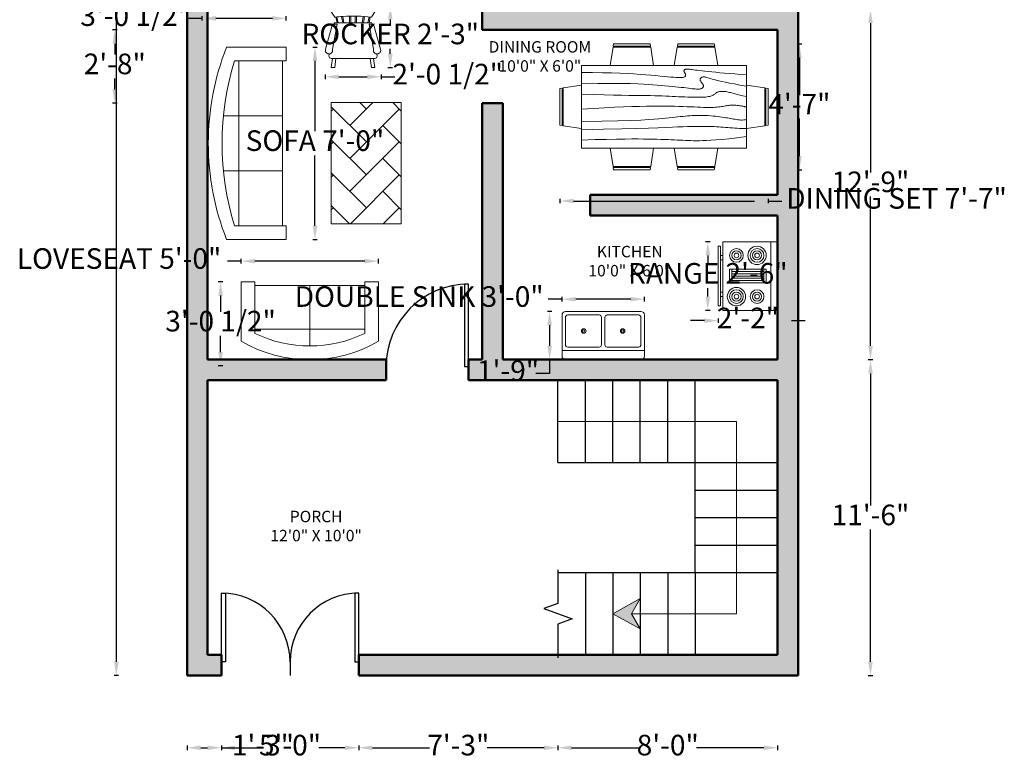
# Model space of a CAD drawing. Units: inches. Extents: x -31 to 401, y -19 to 637.
# Tile 1 of 2: x -29 to 401, y -19 to 305. Entities that reach past the tile are written whole.
import ezdxf

# ---------------------------------------------------------------- set-up
doc = ezdxf.new("R2010")
doc.units = ezdxf.units.IN
for name, color, linetype, lineweight in [('A-ANNO-DIMS', 2, 'Continuous', 18), ('A-ANNO-SYMB', 7, 'Continuous', 18), ('A-AREA-IDEN', 7, 'Continuous', 25), ('A-DOOR', 4, 'Continuous', 25), ('A-EQPM', 8, 'Continuous', 18), ('A-FLOR-FIXT', 9, 'Continuous', 18), ('A-FLOR-STRS', 7, 'Continuous', 25), ('A-FURN', 8, 'Continuous', 18), ('A-FURN-PATT', 9, 'Continuous', 13), ('A-WALL', 7, 'Continuous', 50), ('A-WALL-PATT', 252, 'Continuous', 13)]:
    doc.layers.add(name, color=color, linetype=linetype, lineweight=lineweight)
doc.styles.get("Standard").update_dxf_attribs({"font": 'arial.ttf'})
doc.dimstyles.new('ISO-25', dxfattribs={"dimtxt": 9, "dimasz": 6, "dimexe": 1, "dimexo": 2, "dimtad": 0, "dimtih": 1, "dimtoh": 1, "dimdec": 1, "dimlunit": 3, "dimtxsty": 'Standard', "dimcen": 2.5, "dimadec": 0, "dimazin": 0, "dimtfac": 1, "dimtdec": 1, "dimtmove": 0, "dimatfit": 3, "dimfxl": 1, "dimfxlon": 1, "dimarcsym": 0})

# ---------------------------------------------------------------- blocks, each defined once
blk = doc.blocks.new('*U8')
for p, q in [((0, 0), (0, -6)), ((30, 0), (30, -6))]:
    blk.add_line(p, q)
blk.add_lwpolyline([(0, 0), (0, 30), (1.75, 30), (1.75, 0)], close=True)
blk.add_arc((0, 0), 30, 0, 90)
blk = doc.blocks.new('*U7')
for p, q in [((-30, 0), (-30, -6)), ((0, 0), (0, -6))]:
    blk.add_line(p, q)
blk.add_lwpolyline([(0, 0), (0, 30), (-1.75, 30), (-1.75, 0)], close=True)
blk.add_arc((0, 0), 30, 90, 180)
blk = doc.blocks.new('*U9')
for p, q in [((0, 0), (0, -6)), ((-36, 0), (-36, -6))]:
    blk.add_line(p, q)
blk.add_lwpolyline([(0, 0), (0, 36), (-1.75, 36), (-1.75, 0)], close=True)
blk.add_arc((0, 0), 36, 90, 180)
blk = doc.blocks.new('Sofa - Roundback 7 ft.')
for p, q in [((-12.00002, -32.4421), (-12.00003, -6.5971)), ((11.99997, -32.4421), (11.99998, -6.5971)), ((-36.000027, -34), (-36.000027, -11.4696)), ((35.99998, -34), (35.99998, -11.4696)), ((-35.999844, -13.3819), (35.9998, -13.3819)), ((-36.000027, -32.4421), (35.99998, -32.4421))]:
    blk.add_line(p, q)
for points in [[(-36.000027, -34), (-42.000027, -34), (-42.000027, -8)], [(41.99998, -8), (41.99998, -34), (35.99998, -34)]]:
    blk.add_lwpolyline(points)
for centre, radius, start, end in [((0, -114.25), 114.25, 68.43141, 111.5686), ((-0.00001, -127.1968), 121.1968, 72.72033, 107.2797)]:
    blk.add_arc(centre, radius, start, end)
blk = doc.blocks.new('Chair - Rocking')
for p, q in [((-8, -4.5), (-10, -1.5)), ((-4.5, -7), (-4.96674, -4.19951)), ((-4, -7), (-4.40532, -4.16272)), ((-1.5, -4.05012), (-1.5, -7)), ((-1, -7), (-1, -4.05012)), ((1, -7), (1, -4.04655)), ((1.5, -4.05012), (1.5, -7)), ((4, -7), (4.40187, -4.18694)), ((4.5, -7), (4.96761, -4.19437)), ((8, -4.5), (10, -1.5)), ((-9, -7.5), (-12, -18.49999)), ((-7, -7.5), (-9, -7.5)), ((-9, -18.49999), (-7, -7.5)), ((-8.23428, -6.99939), (-8.3093, -7.47958)), ((-8.23041, -7), (8.23915, -7)), ((-7.5, -4.5), (-7, -7)), ((-6.5, -7), (-7.02225, -4.43)), ((6.5, -7), (7, -4.4057)), ((7.5, -4.5), (7, -7)), ((7, -7.5), (9, -7.5)), ((9, -18.49999), (7, -7.5)), ((8.31071, -7.48854), (8.23449, -7.00073)), ((9, -7.5), (12, -18.49999)), ((-10.36644, -20.64523), (-10.5, -21.49999)), ((10.5, -21.49999), (10.3575, -20.58798)), ((-9, -22.49999), (-9.5, -26.49999)), ((0, -22.49999), (-9.5, -22.49999)), ((-8, -26.49999), (-7.5, -22.49999)), ((0, -22.49999), (9.5, -22.49999)), ((8, -26.49999), (7.5, -22.49999)), ((9, -22.49999), (9.5, -26.49999)), ((-9.5, -26.49999), (-8, -26.49999)), ((9.5, -26.49999), (8, -26.49999))]:
    blk.add_line(p, q)
for centre, radius, start, end in [((0, -34.08333), 34.08333, 72.93847, 107.0615), ((0, -68.25004), 64.25, 93.92211, 97.15267), ((0, -68.25004), 64.25, 82.84733, 93.92211), ((-10.5, -18.99999), 1.58114, 161.5651, 18.43495), ((-9.5, -21.49999), 1, 180, 270), ((10.5, -18.99999), 1.58114, 161.5651, 18.43495), ((9.5, -21.49999), 1, 270, 0)]:
    blk.add_arc(centre, radius, start, end)
blk = doc.blocks.new('Sofa - Roundback Loveseat 5 ft.')
for p, q in [((0, -32.44198), (0, -5.99998)), ((-24, -33.99998), (-24, -11.46958)), ((24.00004, -33.99998), (24.00004, -11.46958)), ((-23.9998, -13.38178), (23.99986, -13.38178)), ((-24, -32.44198), (24.00004, -32.44198))]:
    blk.add_line(p, q)
for points in [[(-24, -33.99998), (-30, -33.99998), (-30, -7.99998)], [(30.00004, -7.99998), (30.00004, -33.99998), (24.00004, -33.99998)]]:
    blk.add_lwpolyline(points)
for centre, radius, start, end in [((0, -60.24998), 60.24998, 60.13715, 119.8628), ((0, -61.38438), 55.38444, 64.32083, 115.6792)]:
    blk.add_arc(centre, radius, start, end)
blk = doc.blocks.new('Dining Set - 36 x 72 in.')
for p, q in [((-22.2343, 26.00059), (-23.4847, 17.99762)), ((-22.2304, 26), (-5.7608, 26)), ((-22, 27.5), (-22.1562, 26.50042)), ((-5.8416, 26.5), (-22.1534, 26.5)), ((-22, 27.5), (-6, 27.5)), ((-5.8437, 26.49966), (-6, 27.5)), ((-4.5152, 17.99762), (-5.7655, 25.99926)), ((5.7657, 26.00059), (4.5153, 17.99762)), ((5.7696, 26), (22.2392, 26)), ((6, 27.5), (5.8438, 26.50042)), ((22.1584, 26.5), (5.8466, 26.5)), ((6, 27.5), (22, 27.5)), ((22.1563, 26.49966), (22, 27.5)), ((23.4848, 17.99762), (22.2345, 25.99926)), ((36, 18), (-36, 18)), ((-36, 18), (-36, -18)), ((36, -18), (36, 18)), ((-44.0006, 8.23428), (-35.9976, 9.48474)), ((44.0006, 8.23428), (35.9976, 9.48474)), ((-45.5, 8), (-44.5004, 8.15617)), ((-45.5, 8), (-45.5, -8)), ((-44.5, -8.15843), (-44.5, 8.15338)), ((-44, 8.23041), (-44, -8.23915)), ((44, 8.23041), (44, -8.23915)), ((44.5, -8.15843), (44.5, 8.15338)), ((45.5, 8), (44.5005, 8.15617)), ((45.5, 8), (45.5, -8)), ((-44.4997, -8.15631), (-45.5, -8)), ((-35.9976, -9.48476), (-43.9993, -8.2345)), ((35.9976, -9.48476), (43.9993, -8.2345)), ((44.4997, -8.15631), (45.5, -8)), ((-36, -18), (36, -18)), ((-22.2343, -26.0006), (-23.4847, -17.99762)), ((-4.5152, -17.99762), (-5.7655, -25.99928)), ((5.7657, -26.0006), (4.5153, -17.99762)), ((23.4848, -17.99762), (22.2345, -25.99928)), ((-22.2304, -26), (-5.7608, -26)), ((-22, -27.5), (-22.1562, -26.50044)), ((-5.8416, -26.5), (-22.1534, -26.5)), ((-22, -27.5), (-6, -27.5)), ((-5.8437, -26.49967), (-6, -27.5)), ((5.7696, -26), (22.2392, -26)), ((6, -27.5), (5.8438, -26.50044)), ((22.1584, -26.5), (5.8466, -26.5)), ((6, -27.5), (22, -27.5)), ((22.1563, -26.49967), (22, -27.5))]:
    blk.add_line(p, q)
for points in [[(-36, 15), (-31.1772, 14.97754), (-26.8079, 14.91406), (-22.8538, 14.81543), (-19.276, 14.6875), (-16.0362, 14.53613), (-13.0957, 14.36718), (-10.4159, 14.18652), (-7.9583, 14), (-5.6904, 13.81315), (-3.6035, 13.63021), (-1.6954, 13.45508), (0.0365, 13.29166), (1.5945, 13.14388), (2.9811, 13.01562), (4.1988, 12.9108), (5.25, 12.83333), (6.1393, 12.78613), (6.8802, 12.76823), (7.4883, 12.77767), (7.9792, 12.8125), (8.3685, 12.87077), (8.6719, 12.95052), (8.9049, 13.0498), (9.0833, 13.16666), (9.2205, 13.29899), (9.3216, 13.44401), (9.3895, 13.59879), (9.4271, 13.76041), (9.4373, 13.92594), (9.4232, 14.09245), (9.3875, 14.257), (9.3333, 14.41666), (9.2638, 14.56917), (9.1836, 14.71484), (9.0975, 14.85465), (9.0104, 14.98958), (8.9272, 15.1206), (8.8529, 15.2487), (8.7922, 15.37483), (8.75, 15.5), (8.7305, 15.62467), (8.7344, 15.74739), (8.7617, 15.86621), (8.8125, 15.97916), (8.8867, 16.08431), (8.9844, 16.17968), (9.1055, 16.26334), (9.25, 16.33333), (9.4189, 16.38802), (9.6172, 16.42708), (9.8506, 16.45052), (10.125, 16.45833), (10.4463, 16.45052), (10.8203, 16.42708), (11.2529, 16.38802), (11.75, 16.33333), (12.3184, 16.26318), (12.9694, 16.17838), (13.7151, 16.07991), (14.5677, 15.96875), (15.5395, 15.84586), (16.6426, 15.71224), (17.8893, 15.56884), (19.2917, 15.41666), (20.859, 15.25667), (22.5879, 15.08984), (24.4721, 14.91715), (26.5052, 14.73958), (28.6809, 14.5581), (30.9929, 14.3737), (33.4347, 14.18733), (36, 14)], [(-36, 10), (-28.9766, 10.14274), (-23.1725, 10.20442), (-18.4241, 10.19775), (-14.5677, 10.13541), (-11.4399, 10.03011), (-8.877, 9.89453), (-6.7154, 9.74137), (-4.7917, 9.58333), (-2.9698, 9.43082), (-1.2246, 9.28515), (0.4415, 9.14534), (2.026, 9.01041), (3.5266, 8.87939), (4.9408, 8.7513), (6.266, 8.62516), (7.5, 8.5), (8.6411, 8.37549), (9.6914, 8.2539), (10.6538, 8.13818), (11.5312, 8.03125), (12.3267, 7.93603), (13.043, 7.85547), (13.6831, 7.79248), (14.25, 7.75), (14.7471, 7.7303), (15.1797, 7.73307), (15.5537, 7.75732), (15.875, 7.80208), (16.1494, 7.86637), (16.3828, 7.94922), (16.5811, 8.04964), (16.75, 8.16666), (16.8944, 8.29915), (17.0143, 8.44531), (17.1089, 8.60319), (17.1771, 8.77083), (17.218, 8.94629), (17.2305, 9.1276), (17.2137, 9.31282), (17.1667, 9.5), (17.0895, 9.6875), (16.987, 9.875), (16.8649, 10.0625), (16.7292, 10.25), (16.5856, 10.4375), (16.4401, 10.625), (16.2985, 10.8125), (16.1667, 11), (16.05, 11.18733), (15.9518, 11.3737), (15.8752, 11.5581), (15.8229, 11.73958), (15.798, 11.91715), (15.8034, 12.08984), (15.842, 12.25667), (15.9167, 12.41666), (16.0295, 12.56836), (16.1784, 12.70833), (16.3605, 12.83268), (16.5729, 12.9375), (16.8127, 13.01888), (17.0768, 13.07291), (17.3625, 13.0957), (17.6667, 13.08333), (17.9894, 13.03312), (18.3418, 12.94726), (18.7382, 12.82918), (19.1927, 12.68229), (19.7195, 12.51001), (20.3327, 12.31575), (21.0465, 12.10294), (21.875, 11.875), (22.8357, 11.63354), (23.959, 11.37304), (25.2786, 11.08618), (26.8282, 10.76562), (28.6414, 10.40405), (30.752, 9.99414), (33.1936, 9.52856), (36, 9)], [(-36, 5.5), (-30.7157, 5.3348), (-26.069, 5.20963), (-21.9946, 5.11767), (-18.4271, 5.05208), (-15.3009, 5.00602), (-12.5508, 4.97265), (-10.1112, 4.94515), (-7.9167, 4.91666), (-5.909, 4.88167), (-4.0586, 4.83984), (-2.3429, 4.79215), (-0.7396, 4.73958), (0.7739, 4.6831), (2.22, 4.6237), (3.6213, 4.56233), (5, 4.5), (6.373, 4.43782), (7.7344, 4.3776), (9.0723, 4.32129), (10.375, 4.27083), (11.6309, 4.22819), (12.8281, 4.19531), (13.9551, 4.17415), (15, 4.16666), (15.954, 4.17448), (16.819, 4.19791), (17.6001, 4.23698), (18.3021, 4.29166), (18.9299, 4.36198), (19.4883, 4.44791), (19.9823, 4.54948), (20.4167, 4.66666), (20.7969, 4.79899), (21.1302, 4.94401), (21.4245, 5.09879), (21.6875, 5.26041), (21.9271, 5.42594), (22.1511, 5.59245), (22.3672, 5.757), (22.5834, 5.91666), (22.8065, 6.06868), (23.0404, 6.21093), (23.2879, 6.34147), (23.5521, 6.45833), (23.8358, 6.55957), (24.142, 6.64323), (24.4735, 6.70735), (24.8334, 6.75), (25.2235, 6.76969), (25.642, 6.76692), (26.0858, 6.74267), (26.5521, 6.69791), (27.0379, 6.63362), (27.5404, 6.55078), (28.0565, 6.45036), (28.5834, 6.33333), (29.1242, 6.19987), (29.7071, 6.04687), (30.3661, 5.87044), (31.1354, 5.66666), (32.0493, 5.43164), (33.142, 5.16146), (34.4475, 4.85221), (36, 4.5)], [(-36, -1), (-30.7915, -0.6591), (-26.0195, -0.38216), (-21.6519, -0.16284), (-17.6563, 0.00521), (-14.0005, 0.12833), (-10.6523, 0.21289), (-7.5796, 0.26522), (-4.75, 0.29166), (-2.134, 0.29793), (0.2878, 0.28711), (2.5317, 0.26163), (4.6146, 0.22396), (6.5529, 0.17651), (8.3633, 0.12174), (10.0623, 0.06209), (11.6667, 0), (13.1899, -0.06201), (14.6341, -0.1211), (15.9982, -0.17432), (17.2813, -0.21875), (18.4823, -0.25147), (19.6003, -0.26953), (20.6343, -0.27002), (21.5834, -0.25), (22.4481, -0.20768), (23.2357, -0.14584), (23.9549, -0.06836), (24.6146, 0.02083), (25.2235, 0.11784), (25.7904, 0.21875), (26.3241, 0.31966), (26.8334, 0.41666), (27.3265, 0.50618), (27.8099, 0.58593), (28.2894, 0.65397), (28.7709, 0.70833), (29.2601, 0.74707), (29.763, 0.76823), (30.2855, 0.76985), (30.8334, 0.75), (31.4088, 0.70784), (31.9994, 0.64713), (32.589, 0.57275), (33.1615, 0.48958), (33.7008, 0.4025), (34.1908, 0.3164), (34.6153, 0.23616), (34.9584, 0.16666), (35.2099, 0.11165), (35.3848, 0.07031), (35.504, 0.04069), (35.5886, 0.02083), (35.6594, 0.00879), (35.7377, 0.0026), (35.8442, 0.00032), (36, 0)], [(-36, -6.5), (-27.1843, -6.31267), (-20.084, -6.1263), (-14.469, -5.9419), (-10.1094, -5.76042), (-6.7752, -5.58285), (-4.2363, -5.41016), (-2.2629, -5.24333), (-0.625, -5.08334), (0.8708, -4.93099), (2.2715, -4.78646), (3.5872, -4.64974), (4.8281, -4.52084), (6.0046, -4.39974), (7.127, -4.28646), (8.2053, -4.18099), (9.25, -4.08334), (10.2705, -3.99382), (11.2734, -3.91407), (12.2647, -3.84603), (13.25, -3.79167), (14.2354, -3.75293), (15.2266, -3.73177), (16.2295, -3.73015), (17.25, -3.75), (18.2912, -3.79248), (19.3451, -3.85547), (20.4009, -3.93604), (21.4479, -4.03125), (22.4754, -4.13819), (23.4727, -4.25391), (24.4289, -4.37549), (25.3334, -4.5), (26.1785, -4.62492), (26.9694, -4.74935), (27.7145, -4.87281), (28.4219, -4.99479), (29.1, -5.11483), (29.7572, -5.23242), (30.4016, -5.34709), (31.0417, -5.45834), (31.6837, -5.56437), (32.3262, -5.65821), (32.9658, -5.73153), (33.599, -5.77604), (34.2224, -5.78345), (34.8327, -5.74545), (35.4264, -5.65373), (36, -5.5)], [(-36, -10), (-26.4022, -9.81299), (-18.4675, -9.62891), (-11.9839, -9.45069), (-6.7396, -9.28125), (-2.5226, -9.12354), (0.8789, -8.98047), (3.6769, -8.85498), (6.0833, -8.75), (8.2767, -8.66765), (10.3021, -8.60677), (12.1712, -8.56543), (13.8958, -8.54167), (15.4876, -8.53353), (16.9583, -8.53907), (18.3197, -8.55632), (19.5834, -8.58334), (20.7616, -8.61841), (21.8685, -8.66081), (22.9188, -8.71004), (23.9271, -8.76563), (24.9081, -8.82707), (25.8763, -8.89388), (26.8465, -8.96558), (27.8334, -9.04167), (28.8474, -9.12118), (29.8828, -9.20117), (30.93, -9.27824), (31.9792, -9.34896), (33.0205, -9.40991), (34.0443, -9.45768), (35.0407, -9.48885), (36, -9.5)], [(-36, -14.5), (-30.0881, -14.33513), (-25.0332, -14.21224), (-20.7312, -14.12647), (-17.0781, -14.07292), (-13.97, -14.04671), (-11.3027, -14.04297), (-8.9724, -14.05681), (-6.875, -14.08334), (-4.9224, -14.11833), (-3.0905, -14.16016), (-1.3709, -14.20785), (0.2448, -14.26042), (1.7647, -14.3169), (3.1973, -14.3763), (4.5507, -14.43767), (5.8333, -14.5), (7.0554, -14.5621), (8.235, -14.62175), (9.3922, -14.67652), (10.5469, -14.72396), (11.7192, -14.76164), (12.929, -14.78711), (14.1965, -14.79794), (15.5417, -14.79167), (16.9933, -14.76424), (18.6152, -14.70508), (20.4804, -14.60197), (22.6615, -14.44271), (25.2312, -14.21509), (28.2624, -13.9069), (31.8277, -13.50594), (36, -13)]]:
    blk.add_lwpolyline(points)
blk = doc.blocks.new('Sink-double - 36 in top')
for p, q in [((-18, -4), (18, -4)), ((-0.75, -18.5), (-0.75, -6.5)), ((0.75, -6.5), (0.75, -18.5))]:
    blk.add_line(p, q)
for points in [[(-16.5, 0), (16.5, 0)], [(-18, -19.5), (-18, -1.5)], [(18, -1.5), (18, -19.5)], [(-16.5, -18.5), (-16.5, -6.5)], [(-15.5, -5.5), (-1.75, -5.5)], [(1.75, -5.5), (15.5, -5.5)], [(16.5, -6.5), (16.5, -18.5)], [(16.5, -21), (-16.5, -21)], [(-1.75, -19.5), (-15.5, -19.5)], [(15.5, -19.5), (1.75, -19.5)]]:
    blk.add_lwpolyline(points)
for centre, radius in [((-8.5, -12.5), 1), ((-8.5, -12.5), 0.5), ((8.5, -12.5), 1), ((8.5, -12.5), 0.5)]:
    blk.add_circle(centre, radius)
for centre, radius, start, end in [((-16.5, -1.5), 1.5, 90, 180), ((16.5, -1.5), 1.5, 0, 90), ((-15.5, -6.5), 1, 90, 180), ((-1.75, -6.5), 1, 0, 90), ((1.75, -6.5), 1, 90, 180), ((15.5, -6.5), 1, 0, 90), ((-16.5, -19.5), 1.5, 180, 270), ((-15.5, -18.5), 1, 180, 270), ((-1.75, -18.5), 1, 270, 0), ((1.75, -18.5), 1, 180, 270), ((15.5, -18.5), 1, 270, 0), ((16.5, -19.5), 1.5, 270, 0)]:
    blk.add_arc(centre, radius, start, end)
blk = doc.blocks.new('Range-Oven - 30 in top')
for p, q in [((0, -3), (30, -3)), ((12, -6), (18, -6)), ((13, -20), (13, -6)), ((14, -6), (14, -20)), ((15, -20), (15, -6)), ((16, -6), (16, -20)), ((17, -20), (17, -6)), ((18, -20), (12, -20)), ((6, -24), (6, -25)), ((8, -25), (8, -24)), ((22, -25), (22, -24)), ((24, -24), (24, -25))]:
    blk.add_line(p, q)
for points in [[(0, -24), (0, 0), (30, 0), (30, -24)], [(12, -21), (12, -5), (18, -5), (18, -21)], [(2, -26), (2, -25), (28, -25), (28, -26)]]:
    blk.add_lwpolyline(points, close=True)
for centre, radius in [((6, -9), 4), ((6, -9), 3), ((6, -9), 2), ((6, -9), 1), ((24, -9), 3), ((24, -9), 2), ((24, -9), 1), ((6, -18), 3), ((6, -18), 2), ((6, -18), 1), ((24, -18), 4), ((24, -18), 3), ((24, -18), 2), ((24, -18), 1)]:
    blk.add_circle(centre, radius)
blk = doc.blocks.new('*D20')
at = {"layer": 'A-ANNO-DIMS', "color": 0, "lineweight": -2, "transparency": 16777216}
for p, q in [((13.91, 618.38), (11.91, 618.38)), ((12.91, 612.38), (12.91, 323.6)), ((12.91, 24.38), (12.91, 313.16)), ((13.91, 18.38), (11.91, 18.38))]:
    blk.add_line(p, q, dxfattribs=at)
at = {"layer": 'A-ANNO-DIMS', "color": 0, "transparency": 16777216}
for points in [[(11.91, 612.38), (13.91, 612.38), (12.91, 618.38)], [(11.91, 24.38), (13.91, 24.38), (12.91, 18.38)]]:
    blk.add_solid(points, dxfattribs=at)
at = {"layer": 'Defpoints', "color": 0, "transparency": 16777216}
for p in [(43.78, 618.38), (12.91, 18.38), (43.78, 18.38)]:
    blk.add_point(p, dxfattribs=at)
at = {"layer": 'A-ANNO-DIMS', "color": 0, "transparency": 16777216, "insert": (12.91, 318.38), "char_height": 9, "attachment_point": 5}
blk.add_mtext("50'", dxfattribs=at)
blk = doc.blocks.new('*D28')
at = {"layer": 'A-ANNO-DIMS', "color": 0, "lineweight": -2, "transparency": 16777216}
for p, q in [((98.67, 292.87), (100.67, 292.87)), ((99.67, 286.87), (99.67, 256.16)), ((99.67, 214.87), (99.67, 245.59)), ((98.67, 208.87), (100.67, 208.87))]:
    blk.add_line(p, q, dxfattribs=at)
at = {"layer": 'A-ANNO-DIMS', "color": 0, "transparency": 16777216}
for points in [[(98.67, 286.87), (100.67, 286.87), (99.67, 292.87)], [(98.67, 214.87), (100.67, 214.87), (99.67, 208.87)]]:
    blk.add_solid(points, dxfattribs=at)
at = {"layer": 'Defpoints', "color": 0, "transparency": 16777216}
for p in [(87.07, 292.87), (99.67, 292.87), (87.07, 208.87)]:
    blk.add_point(p, dxfattribs=at)
at = {"layer": 'A-ANNO-DIMS', "color": 0, "transparency": 16777216, "insert": (99.67, 250.87), "char_height": 9, "attachment_point": 5}
blk.add_mtext('SOFA 7\'-0"', dxfattribs=at)
blk = doc.blocks.new('*D29')
at = {"layer": 'A-ANNO-DIMS', "color": 0, "lineweight": -2, "transparency": 16777216}
for p, q in [((50.4, 305.47), (44.4, 305.47)), ((50.4, 304.47), (50.4, 306.47)), ((81.07, 305.47), (56.4, 305.47)), ((87.07, 304.47), (87.07, 306.47))]:
    blk.add_line(p, q, dxfattribs=at)
at = {"layer": 'A-ANNO-DIMS', "color": 0, "transparency": 16777216}
for points in [[(56.4, 306.47), (56.4, 304.47), (50.4, 305.47)], [(81.07, 306.47), (81.07, 304.47), (87.07, 305.47)]]:
    blk.add_solid(points, dxfattribs=at)
at = {"layer": 'Defpoints', "color": 0, "transparency": 16777216}
for p in [(50.4, 305.47), (50.4, 292.87), (87.07, 292.87)]:
    blk.add_point(p, dxfattribs=at)
at = {"layer": 'A-ANNO-DIMS', "color": 0, "transparency": 16777216, "insert": (21.33, 305.47), "char_height": 9, "attachment_point": 5}
blk.add_mtext('3\'-0 1/2"', dxfattribs=at)
blk = doc.blocks.new('*D30')
at = {"layer": 'A-ANNO-DIMS', "color": 0, "lineweight": -2, "transparency": 16777216}
for p, q in [((131.57, 310.98), (133.57, 310.98)), ((132.57, 304.98), (132.57, 302.76)), ((132.57, 289.98), (132.57, 292.19)), ((131.57, 283.98), (133.57, 283.98))]:
    blk.add_line(p, q, dxfattribs=at)
at = {"layer": 'A-ANNO-DIMS', "color": 0, "transparency": 16777216}
for points in [[(131.57, 304.98), (133.57, 304.98), (132.57, 310.98)], [(131.57, 289.98), (133.57, 289.98), (132.57, 283.98)]]:
    blk.add_solid(points, dxfattribs=at)
at = {"layer": 'Defpoints', "color": 0, "transparency": 16777216}
for p in [(128.52, 310.98), (132.57, 310.98), (128.52, 283.98)]:
    blk.add_point(p, dxfattribs=at)
at = {"layer": 'A-ANNO-DIMS', "color": 0, "transparency": 16777216, "insert": (132.57, 297.48), "char_height": 9, "attachment_point": 5}
blk.add_mtext('ROCKER 2\'-3"', dxfattribs=at)
blk = doc.blocks.new('*D31')
at = {"layer": 'A-ANNO-DIMS', "color": 0, "lineweight": -2, "transparency": 16777216}
for p, q in [((104.09, 280.93), (104.09, 278.93)), ((110.09, 279.93), (122.52, 279.93)), ((128.52, 280.93), (128.52, 278.93)), ((128.52, 279.93), (134.52, 279.93))]:
    blk.add_line(p, q, dxfattribs=at)
at = {"layer": 'A-ANNO-DIMS', "color": 0, "transparency": 16777216}
for points in [[(110.09, 280.93), (110.09, 278.93), (104.09, 279.93)], [(122.52, 280.93), (122.52, 278.93), (128.52, 279.93)]]:
    blk.add_solid(points, dxfattribs=at)
at = {"layer": 'Defpoints', "color": 0, "transparency": 16777216}
for p in [(104.09, 283.98), (128.52, 283.98), (128.52, 279.93)]:
    blk.add_point(p, dxfattribs=at)
at = {"layer": 'A-ANNO-DIMS', "color": 0, "transparency": 16777216, "insert": (157.67, 279.93), "char_height": 9, "attachment_point": 5}
blk.add_mtext('2\'-0 1/2"', dxfattribs=at)
blk = doc.blocks.new('*D32')
at = {"layer": 'A-ANNO-DIMS', "color": 0, "lineweight": -2, "transparency": 16777216}
for p, q in [((67.44, 199.38), (61.44, 199.38)), ((67.44, 198.38), (67.44, 200.38)), ((121.44, 199.38), (73.44, 199.38)), ((127.44, 198.38), (127.44, 200.38))]:
    blk.add_line(p, q, dxfattribs=at)
at = {"layer": 'A-ANNO-DIMS', "color": 0, "transparency": 16777216}
for points in [[(73.44, 200.38), (73.44, 198.38), (67.44, 199.38)], [(121.44, 200.38), (121.44, 198.38), (127.44, 199.38)]]:
    blk.add_solid(points, dxfattribs=at)
at = {"layer": 'Defpoints', "color": 0, "transparency": 16777216}
for p in [(67.44, 199.38), (67.44, 190.38), (127.44, 190.38)]:
    blk.add_point(p, dxfattribs=at)
at = {"layer": 'A-ANNO-DIMS', "color": 0, "transparency": 16777216, "insert": (14.11, 199.38), "char_height": 9, "attachment_point": 5}
blk.add_mtext('LOVESEAT 5\'-0"', dxfattribs=at)
blk = doc.blocks.new('*D33')
at = {"layer": 'A-ANNO-DIMS', "color": 0, "lineweight": -2, "transparency": 16777216}
for p, q in [((59.44, 190.38), (57.44, 190.38)), ((58.44, 184.38), (58.44, 177.33)), ((58.44, 159.71), (58.44, 166.76)), ((59.44, 153.71), (57.44, 153.71))]:
    blk.add_line(p, q, dxfattribs=at)
at = {"layer": 'A-ANNO-DIMS', "color": 0, "transparency": 16777216}
for points in [[(57.44, 184.38), (59.44, 184.38), (58.44, 190.38)], [(57.44, 159.71), (59.44, 159.71), (58.44, 153.71)]]:
    blk.add_solid(points, dxfattribs=at)
at = {"layer": 'Defpoints', "color": 0, "transparency": 16777216}
for p in [(67.44, 190.38), (58.44, 153.71), (67.44, 153.71)]:
    blk.add_point(p, dxfattribs=at)
at = {"layer": 'A-ANNO-DIMS', "color": 0, "transparency": 16777216, "insert": (58.44, 172.04), "char_height": 9, "attachment_point": 5}
blk.add_mtext('3\'-0 1/2"', dxfattribs=at)
blk = doc.blocks.new('*D34')
at = {"layer": 'A-ANNO-DIMS', "color": 0, "lineweight": -2, "transparency": 16777216}
for p, q in [((206.62, 226.66), (206.62, 224.66)), ((212.62, 225.66), (291.62, 225.66)), ((297.62, 226.66), (297.62, 224.66)), ((297.62, 225.66), (303.62, 225.66))]:
    blk.add_line(p, q, dxfattribs=at)
at = {"layer": 'A-ANNO-DIMS', "color": 0, "transparency": 16777216}
for points in [[(212.62, 226.66), (212.62, 224.66), (206.62, 225.66)], [(291.62, 226.66), (291.62, 224.66), (297.62, 225.66)]]:
    blk.add_solid(points, dxfattribs=at)
at = {"layer": 'Defpoints', "color": 0, "transparency": 16777216}
for p in [(206.62, 239.31), (297.62, 239.31), (297.62, 225.66)]:
    blk.add_point(p, dxfattribs=at)
at = {"layer": 'A-ANNO-DIMS', "color": 0, "transparency": 16777216, "insert": (353.71, 225.66), "char_height": 9, "attachment_point": 5}
blk.add_mtext('DINING SET 7\'-7"', dxfattribs=at)
blk = doc.blocks.new('*D35')
at = {"layer": 'A-ANNO-DIMS', "color": 0, "lineweight": -2, "transparency": 16777216}
for p, q in [((310.27, 294.31), (312.27, 294.31)), ((311.27, 288.31), (311.27, 271.93)), ((311.27, 245.31), (311.27, 261.68)), ((310.27, 239.31), (312.27, 239.31))]:
    blk.add_line(p, q, dxfattribs=at)
at = {"layer": 'A-ANNO-DIMS', "color": 0, "transparency": 16777216}
for points in [[(310.27, 288.31), (312.27, 288.31), (311.27, 294.31)], [(310.27, 245.31), (312.27, 245.31), (311.27, 239.31)]]:
    blk.add_solid(points, dxfattribs=at)
at = {"layer": 'Defpoints', "color": 0, "transparency": 16777216}
for p in [(297.62, 294.31), (311.27, 294.31), (297.62, 239.31)]:
    blk.add_point(p, dxfattribs=at)
at = {"layer": 'A-ANNO-DIMS', "color": 0, "transparency": 16777216, "insert": (311.27, 266.81), "char_height": 9, "attachment_point": 5}
blk.add_mtext('4\'-7"', dxfattribs=at)
blk = doc.blocks.new('*D36')
at = {"layer": 'A-ANNO-DIMS', "color": 0, "lineweight": -2, "transparency": 16777216}
for p, q in [((207.58, 182.78), (201.58, 182.78)), ((207.58, 181.78), (207.58, 183.78)), ((237.58, 182.78), (213.58, 182.78)), ((243.58, 181.78), (243.58, 183.78))]:
    blk.add_line(p, q, dxfattribs=at)
at = {"layer": 'A-ANNO-DIMS', "color": 0, "transparency": 16777216}
for points in [[(213.58, 183.78), (213.58, 181.78), (207.58, 182.78)], [(237.58, 183.78), (237.58, 181.78), (243.58, 182.78)]]:
    blk.add_solid(points, dxfattribs=at)
at = {"layer": 'Defpoints', "color": 0, "transparency": 16777216}
for p in [(207.58, 182.78), (207.58, 177.38), (243.58, 177.38)]:
    blk.add_point(p, dxfattribs=at)
at = {"layer": 'A-ANNO-DIMS', "color": 0, "transparency": 16777216, "insert": (145.2, 182.78), "char_height": 9, "attachment_point": 5}
blk.add_mtext('DOUBLE SINK 3\'-0"', dxfattribs=at)
blk = doc.blocks.new('*D37')
at = {"layer": 'A-ANNO-DIMS', "color": 0, "lineweight": -2, "transparency": 16777216}
for p, q in [((203.18, 177.38), (201.18, 177.38)), ((202.18, 171.38), (202.18, 162.38)), ((203.18, 156.38), (201.18, 156.38)), ((202.18, 156.38), (202.18, 150.38)), ((202.18, 150.38), (196.18, 150.38))]:
    blk.add_line(p, q, dxfattribs=at)
at = {"layer": 'A-ANNO-DIMS', "color": 0, "transparency": 16777216}
for points in [[(201.18, 171.38), (203.18, 171.38), (202.18, 177.38)], [(201.18, 162.38), (203.18, 162.38), (202.18, 156.38)]]:
    blk.add_solid(points, dxfattribs=at)
at = {"layer": 'Defpoints', "color": 0, "transparency": 16777216}
for p in [(207.58, 177.38), (202.18, 156.38), (207.58, 156.38)]:
    blk.add_point(p, dxfattribs=at)
at = {"layer": 'A-ANNO-DIMS', "color": 0, "transparency": 16777216, "insert": (184.02, 150.38), "char_height": 9, "attachment_point": 5}
blk.add_mtext('1\'-9"', dxfattribs=at)
blk = doc.blocks.new('*D38')
at = {"layer": 'A-ANNO-DIMS', "color": 0, "lineweight": -2, "transparency": 16777216}
for p, q in [((272.28, 207.91), (270.28, 207.91)), ((271.28, 201.91), (271.28, 198.19)), ((271.28, 183.91), (271.28, 187.63)), ((272.28, 177.91), (270.28, 177.91))]:
    blk.add_line(p, q, dxfattribs=at)
at = {"layer": 'A-ANNO-DIMS', "color": 0, "transparency": 16777216}
for points in [[(270.28, 201.91), (272.28, 201.91), (271.28, 207.91)], [(270.28, 183.91), (272.28, 183.91), (271.28, 177.91)]]:
    blk.add_solid(points, dxfattribs=at)
at = {"layer": 'Defpoints', "color": 0, "transparency": 16777216}
for p in [(275.78, 207.91), (271.28, 177.91), (275.78, 177.91)]:
    blk.add_point(p, dxfattribs=at)
at = {"layer": 'A-ANNO-DIMS', "color": 0, "transparency": 16777216, "insert": (271.28, 192.91), "char_height": 9, "attachment_point": 5}
blk.add_mtext('RANGE 2\'-6"', dxfattribs=at)
blk = doc.blocks.new('*D39')
at = {"layer": 'A-ANNO-DIMS', "color": 0, "lineweight": -2, "transparency": 16777216}
for p, q in [((269.78, 173.41), (263.78, 173.41)), ((275.78, 174.41), (275.78, 172.41)), ((275.78, 173.41), (276.12, 173.41)), ((301.78, 173.41), (301.45, 173.41)), ((301.78, 174.41), (301.78, 172.41)), ((307.78, 173.41), (313.78, 173.41))]:
    blk.add_line(p, q, dxfattribs=at)
at = {"layer": 'A-ANNO-DIMS', "color": 0, "transparency": 16777216}
for points in [[(269.78, 174.41), (269.78, 172.41), (275.78, 173.41)], [(307.78, 174.41), (307.78, 172.41), (301.78, 173.41)]]:
    blk.add_solid(points, dxfattribs=at)
at = {"layer": 'Defpoints', "color": 0, "transparency": 16777216}
for p in [(275.78, 177.91), (301.78, 177.91), (301.78, 173.41)]:
    blk.add_point(p, dxfattribs=at)
at = {"layer": 'A-ANNO-DIMS', "color": 0, "transparency": 16777216, "insert": (288.78, 173.41), "char_height": 9, "attachment_point": 5}
blk.add_mtext('2\'-2"', dxfattribs=at)
blk = doc.blocks.new('*D40')
at = {"layer": 'A-ANNO-DIMS', "color": 0, "lineweight": -2, "transparency": 16777216}
for p, q in [((43.78, -12.17), (43.78, -14.17)), ((58.78, -12.17), (58.78, -14.17)), ((49.78, -13.17), (52.78, -13.17)), ((58.78, -13.17), (64.78, -13.17))]:
    blk.add_line(p, q, dxfattribs=at)
at = {"layer": 'A-ANNO-DIMS', "color": 0, "transparency": 16777216}
for points in [[(49.78, -12.17), (49.78, -14.17), (43.78, -13.17)], [(52.78, -12.17), (52.78, -14.17), (58.78, -13.17)]]:
    blk.add_solid(points, dxfattribs=at)
at = {"layer": 'Defpoints', "color": 0, "transparency": 16777216}
for p in [(43.78, 18.38), (58.78, 18.38), (58.78, -13.17)]:
    blk.add_point(p, dxfattribs=at)
at = {"layer": 'A-ANNO-DIMS', "color": 0, "transparency": 16777216, "insert": (76.95, -13.17), "char_height": 9, "attachment_point": 5}
blk.add_mtext('1\'-3"', dxfattribs=at)
blk = doc.blocks.new('*D41')
at = {"layer": 'A-ANNO-DIMS', "color": 0, "lineweight": -2, "transparency": 16777216}
for p, q in [((58.78, -12.17), (58.78, -14.17)), ((118.78, -12.17), (118.78, -14.17)), ((64.78, -13.17), (76.2, -13.17)), ((112.78, -13.17), (101.37, -13.17))]:
    blk.add_line(p, q, dxfattribs=at)
at = {"layer": 'A-ANNO-DIMS', "color": 0, "transparency": 16777216}
for points in [[(64.78, -12.17), (64.78, -14.17), (58.78, -13.17)], [(112.78, -12.17), (112.78, -14.17), (118.78, -13.17)]]:
    blk.add_solid(points, dxfattribs=at)
at = {"layer": 'Defpoints', "color": 0, "transparency": 16777216}
for p in [(58.78, 18.38), (118.78, 18.38), (118.78, -13.17)]:
    blk.add_point(p, dxfattribs=at)
at = {"layer": 'A-ANNO-DIMS', "color": 0, "transparency": 16777216, "insert": (88.78, -13.17), "char_height": 9, "attachment_point": 5}
blk.add_mtext('5\'-0"', dxfattribs=at)
blk = doc.blocks.new('*D42')
at = {"layer": 'A-ANNO-DIMS', "color": 0, "lineweight": -2, "transparency": 16777216}
for p, q in [((118.78, -12.17), (118.78, -14.17)), ((205.78, -12.17), (205.78, -14.17)), ((124.78, -13.17), (149.73, -13.17)), ((199.78, -13.17), (174.83, -13.17))]:
    blk.add_line(p, q, dxfattribs=at)
at = {"layer": 'A-ANNO-DIMS', "color": 0, "transparency": 16777216}
for points in [[(124.78, -12.17), (124.78, -14.17), (118.78, -13.17)], [(199.78, -12.17), (199.78, -14.17), (205.78, -13.17)]]:
    blk.add_solid(points, dxfattribs=at)
at = {"layer": 'Defpoints', "color": 0, "transparency": 16777216}
for p in [(205.78, 26.13), (118.78, 18.38), (205.78, -13.17)]:
    blk.add_point(p, dxfattribs=at)
at = {"layer": 'A-ANNO-DIMS', "color": 0, "transparency": 16777216, "insert": (162.28, -13.17), "char_height": 9, "attachment_point": 5}
blk.add_mtext('7\'-3"', dxfattribs=at)
blk = doc.blocks.new('*D43')
at = {"layer": 'A-ANNO-DIMS', "color": 0, "lineweight": -2, "transparency": 16777216}
for p, q in [((205.78, -12.17), (205.78, -14.17)), ((301.78, -12.17), (301.78, -14.17)), ((211.78, -13.17), (241.19, -13.17)), ((295.78, -13.17), (266.38, -13.17))]:
    blk.add_line(p, q, dxfattribs=at)
at = {"layer": 'A-ANNO-DIMS', "color": 0, "transparency": 16777216}
for points in [[(211.78, -12.17), (211.78, -14.17), (205.78, -13.17)], [(295.78, -12.17), (295.78, -14.17), (301.78, -13.17)]]:
    blk.add_solid(points, dxfattribs=at)
at = {"layer": 'Defpoints', "color": 0, "transparency": 16777216}
for p in [(205.78, 26.13), (301.78, 27.38), (301.78, -13.17)]:
    blk.add_point(p, dxfattribs=at)
at = {"layer": 'A-ANNO-DIMS', "color": 0, "transparency": 16777216, "insert": (253.78, -13.17), "char_height": 9, "attachment_point": 5}
blk.add_mtext('8\'-0"', dxfattribs=at)
blk = doc.blocks.new('*D44')
at = {"layer": 'A-ANNO-DIMS', "color": 0, "lineweight": -2, "transparency": 16777216}
for p, q in [((341.33, 156.38), (343.33, 156.38)), ((342.33, 150.38), (342.33, 92.6)), ((342.33, 24.38), (342.33, 82.16)), ((341.33, 18.38), (343.33, 18.38))]:
    blk.add_line(p, q, dxfattribs=at)
at = {"layer": 'A-ANNO-DIMS', "color": 0, "transparency": 16777216}
for points in [[(341.33, 150.38), (343.33, 150.38), (342.33, 156.38)], [(341.33, 24.38), (343.33, 24.38), (342.33, 18.38)]]:
    blk.add_solid(points, dxfattribs=at)
at = {"layer": 'Defpoints', "color": 0, "transparency": 16777216}
for p in [(301.78, 156.38), (342.33, 156.38), (310.78, 18.38)]:
    blk.add_point(p, dxfattribs=at)
at = {"layer": 'A-ANNO-DIMS', "color": 0, "transparency": 16777216, "insert": (342.33, 87.38), "char_height": 9, "attachment_point": 5}
blk.add_mtext('11\'-6"', dxfattribs=at)
blk = doc.blocks.new('*D45')
at = {"layer": 'A-ANNO-DIMS', "color": 0, "lineweight": -2, "transparency": 16777216}
for p, q in [((341.33, 309.38), (343.33, 309.38)), ((342.33, 303.38), (342.33, 238.1)), ((342.33, 162.38), (342.33, 227.66)), ((341.33, 156.38), (343.33, 156.38))]:
    blk.add_line(p, q, dxfattribs=at)
at = {"layer": 'A-ANNO-DIMS', "color": 0, "transparency": 16777216}
for points in [[(341.33, 303.38), (343.33, 303.38), (342.33, 309.38)], [(341.33, 162.38), (343.33, 162.38), (342.33, 156.38)]]:
    blk.add_solid(points, dxfattribs=at)
at = {"layer": 'Defpoints', "color": 0, "transparency": 16777216}
for p in [(301.78, 309.38), (342.33, 309.38), (301.78, 156.38)]:
    blk.add_point(p, dxfattribs=at)
at = {"layer": 'A-ANNO-DIMS', "color": 0, "transparency": 16777216, "insert": (342.33, 232.88), "char_height": 9, "attachment_point": 5}
blk.add_mtext('12\'-9"', dxfattribs=at)
blk = doc.blocks.new('*D50')
at = {"layer": 'A-ANNO-DIMS', "color": 0, "lineweight": -2, "transparency": 16777216}
for p, q in [((13.23, 300.38), (11.23, 300.38)), ((12.23, 294.38), (12.23, 289.62)), ((12.23, 274.42), (12.23, 279.18)), ((13.23, 268.42), (11.23, 268.42))]:
    blk.add_line(p, q, dxfattribs=at)
at = {"layer": 'A-ANNO-DIMS', "color": 0, "transparency": 16777216}
for points in [[(11.23, 294.38), (13.23, 294.38), (12.23, 300.38)], [(11.23, 274.42), (13.23, 274.42), (12.23, 268.42)]]:
    blk.add_solid(points, dxfattribs=at)
at = {"layer": 'Defpoints', "color": 0, "transparency": 16777216}
for p in [(12.23, 300.38), (172.78, 300.38), (172.78, 268.42)]:
    blk.add_point(p, dxfattribs=at)
at = {"layer": 'A-ANNO-DIMS', "color": 0, "transparency": 16777216, "insert": (12.23, 284.4), "char_height": 9, "attachment_point": 5}
blk.add_mtext('2\'-8"', dxfattribs=at)

msp = doc.modelspace()

# ---------------------------------------------------------------- hatches: boundary and pattern name
at = {"layer": 'A-ANNO-SYMB'}
h = msp.add_hatch(color=256, dxfattribs=at)
h.dxf.hatch_style = 1
h.paths.add_polyline_path([(237.94, 45.38), (241.78, 52.03), (229.78, 45.38), (241.78, 38.72)])
at = {"layer": 'A-FURN-PATT'}
h = msp.add_hatch(dxfattribs=at)
h.set_pattern_fill('AR-HBONE', color=256, scale=0.1)
h.paths.add_polyline_path([(137.37, 268.64), (106.81, 268.64), (106.81, 215.71), (137.37, 215.71)])
at = {"layer": 'A-WALL-PATT'}
h = msp.add_hatch(color=256, dxfattribs=at)
h.dxf.hatch_style = 1
h.paths.add_polyline_path([(310.78, 618.38), (43.78, 618.38), (43.78, 18.38), (58.78, 18.38), (58.78, 24.38), (58.78, 27.38), (52.78, 27.38), (52.78, 147.38), (130.78, 147.38), (130.78, 153.38), (130.78, 156.38), (52.78, 156.38), (52.78, 361.38), (100.78, 361.38), (100.78, 367.38), (52.78, 367.38), (52.78, 415.38), (126.78, 415.38), (126.78, 430.38), (120.78, 430.38), (120.78, 424.38), (52.78, 424.38), (52.78, 484.38), (120.78, 484.38), (120.78, 462.38), (126.78, 462.38), (126.78, 493.38), (52.78, 493.38), (52.78, 609.38), (172.78, 609.38), (172.78, 493.38), (166.78, 493.38), (166.78, 490.38), (166.78, 484.38), (187.81, 484.38), (187.81, 490.38), (187.81, 493.38), (181.78, 493.38), (181.78, 609.38), (301.78, 609.38), (301.78, 493.38), (277.78, 493.38), (277.78, 487.38), (277.78, 484.38), (301.78, 484.38), (301.78, 424.38), (233.78, 424.38), (233.78, 484.38), (245.78, 484.38), (245.78, 487.38), (245.78, 493.38), (227.78, 493.38), (227.78, 491.76, -0.008619), (227.81, 490.38), (227.81, 484.38), (227.78, 424.38), (222.78, 424.38), (222.78, 418.38), (222.78, 415.38), (301.78, 415.38), (301.78, 309.38), (181.78, 309.38), (181.78, 415.38), (186.78, 415.38), (186.78, 418.38), (186.78, 424.38), (172.78, 424.38), (172.78, 300.38), (301.78, 300.38), (301.78, 228.38), (219.84, 228.38), (219.84, 219.38), (301.78, 219.38), (301.78, 156.38), (181.78, 156.38), (181.78, 219.38), (181.78, 268.42), (172.78, 268.42), (172.78, 156.38), (166.78, 156.38), (166.78, 153.38), (166.78, 147.38), (301.78, 147.38), (301.78, 27.38), (118.78, 27.38), (118.78, 24.38), (118.78, 18.38), (310.78, 18.38)])

# ---------------------------------------------------------------- linework, layer by layer
at = {"layer": 'A-ANNO-SYMB'}
for p, q in [((205.78, 129.38), (283.78, 129.38)), ((283.78, 129.38), (283.78, 45.38)), ((229.78, 45.38), (241.78, 52.03)), ((241.78, 52.03), (237.94, 45.38)), ((229.78, 45.38), (241.78, 38.72)), ((283.78, 45.38), (237.94, 45.38)), ((241.78, 38.72), (237.94, 45.38))]:
    msp.add_line(p, q, dxfattribs=at)
at = {"layer": 'A-FLOR-STRS'}
for p, q in [((205.78, 111.38), (205.78, 147.38)), ((217.78, 111.38), (217.78, 147.38)), ((229.78, 111.38), (229.78, 147.38)), ((241.78, 111.38), (241.78, 147.38)), ((253.78, 111.38), (253.78, 147.38)), ((265.78, 111.38), (265.78, 147.38)), ((205.78, 111.38), (265.78, 111.38)), ((265.78, 63.38), (265.78, 111.38)), ((265.78, 111.38), (301.78, 111.38)), ((265.78, 99.38), (301.78, 99.38)), ((265.78, 87.38), (301.78, 87.38)), ((265.78, 75.38), (301.78, 75.38)), ((205.78, 63.38), (265.78, 63.38)), ((217.78, 63.38), (217.78, 27.38)), ((229.78, 63.38), (229.78, 27.38)), ((241.78, 63.38), (241.78, 27.38)), ((253.78, 63.38), (253.78, 27.38)), ((265.78, 63.38), (301.78, 63.38)), ((265.78, 63.38), (265.78, 27.38))]:
    msp.add_line(p, q, dxfattribs=at)
msp.add_lwpolyline([(205.78, 64.63), (205.78, 49.88), (199.6, 47.63), (211.97, 43.13), (205.78, 40.88), (205.78, 26.13)], dxfattribs=at)
at = {"layer": 'A-FURN'}
msp.add_lwpolyline([(106.81, 268.64), (137.37, 268.64), (137.37, 215.71), (106.81, 215.71)], close=True, dxfattribs=at)
at = {"layer": 'A-WALL'}
for p, q in [((43.78, 618.38), (43.78, 18.38)), ((310.78, 18.38), (310.78, 618.38)), ((172.78, 300.38), (172.78, 424.38)), ((52.78, 361.38), (52.78, 156.38)), ((172.78, 300.38), (301.78, 300.38)), ((301.78, 228.38), (301.78, 300.38)), ((172.78, 156.38), (172.78, 268.42)), ((172.78, 268.42), (181.78, 268.42)), ((181.78, 219.38), (181.78, 268.42)), ((181.78, 264.38), (181.78, 264.38)), ((219.84, 228.38), (301.78, 228.38)), ((219.84, 228.38), (219.84, 219.38)), ((181.78, 156.38), (181.78, 219.38)), ((219.84, 219.38), (301.78, 219.38)), ((301.78, 156.38), (301.78, 219.38)), ((52.78, 156.38), (130.78, 156.38)), ((130.78, 156.38), (130.78, 147.38)), ((166.78, 156.38), (166.78, 147.38)), ((166.78, 156.38), (172.78, 156.38)), ((181.78, 156.38), (301.78, 156.38)), ((52.78, 147.38), (130.78, 147.38)), ((52.78, 147.38), (52.78, 27.38)), ((166.78, 147.38), (301.78, 147.38)), ((301.78, 27.38), (301.78, 147.38)), ((52.78, 27.38), (58.78, 27.38)), ((58.78, 27.38), (58.78, 18.38)), ((118.78, 27.38), (118.78, 18.38)), ((118.78, 27.38), (301.78, 27.38)), ((43.78, 18.38), (58.78, 18.38)), ((118.78, 18.38), (310.78, 18.38))]:
    msp.add_line(p, q, dxfattribs=at)

# ---------------------------------------------------------------- block references
at = {"layer": 'A-DOOR'}
for name, p in [('*U9', (166.78, 153.38)), ('*U8', (58.78, 24.38)), ('*U7', (118.78, 24.38))]:
    msp.add_blockref(name, p, dxfattribs=at)
at = {"layer": 'A-EQPM', "rotation": 270}
msp.add_blockref('Range-Oven - 30 in top', (301.78, 207.91), dxfattribs=at)
at = {"layer": 'A-FLOR-FIXT', "rotation": 180}
msp.add_blockref('Sink-double - 36 in top', (225.58, 156.38), dxfattribs=at)
at = {"layer": 'A-FURN'}
for name, p in [('Chair - Rocking', (116.3, 310.48)), ('Dining Set - 36 x 72 in.', (252.12, 266.81))]:
    msp.add_blockref(name, p, dxfattribs=at)
for name, p, rotation in [('Sofa - Roundback 7 ft.', (53.07, 250.87), 90), ('Sofa - Roundback Loveseat 5 ft.', (97.44, 156.38), 180)]:
    msp.add_blockref(name, p, dxfattribs=dict(at, rotation=rotation))

# ---------------------------------------------------------------- texts
at = {"layer": 'A-AREA-IDEN', "char_height": 5, "attachment_point": 1}
for s, width, insert in [('\\pxqc;DINING ROOM\\P10\'0" X 6\'0"', 52.2741, (171.77, 295.5)), ('\\pxqc;KITCHEN\\P10\'0" X 6\'0"', 40.9025, (216.74, 206.08)), ('\\pxqc;PORCH\\P12\'0" X 10\'0"', 40.9025, (79.74, 90.36))]:
    msp.add_mtext_dynamic_manual_height_columns(s, width=width, gutter_width=12.5, heights=[0], dxfattribs=dict(at, insert=insert))

# ---------------------------------------------------------------- dimensions: what is measured, and where the dimension line sits
at = {"layer": 'A-ANNO-DIMS'}
for base, p1, p2, angle, override, picture, middle in [((12.91, 18.38), (43.78, 618.38), (43.78, 18.38), 90, {"dimclrd": 0, "dimclre": 0, "dimclrt": 0}, '*D20', (12.91, 318.38)), ((50.4, 305.47), (87.07, 292.87), (50.4, 292.87), 180, {"dimdec": 1, "dimlfac": 1, "dimrnd": 0, "dimzin": 1, "dimdsep": 46, "dimlunit": 4, "dimfrac": 2}, '*D29', (21.33, 305.47)), ((342.33, 309.38), (301.78, 156.38), (301.78, 309.38), 90, {"dimdec": 1, "dimlfac": 1, "dimrnd": 0, "dimzin": 1, "dimdsep": 46, "dimlunit": 4, "dimfrac": 2}, '*D45', (342.33, 232.88)), ((12.23, 300.38), (172.78, 268.42), (172.78, 300.38), 90, {"dimdec": 1, "dimlfac": 1, "dimrnd": 0, "dimzin": 1, "dimdsep": 46, "dimlunit": 4, "dimfrac": 2}, '*D50', (12.23, 284.4)), ((311.27, 294.31), (297.62, 239.31), (297.62, 294.31), 90, {"dimdec": 1, "dimlfac": 1, "dimrnd": 0, "dimzin": 1, "dimdsep": 46, "dimlunit": 4, "dimfrac": 2}, '*D35', (311.27, 266.81)), ((58.44, 153.71), (67.44, 190.38), (67.44, 153.71), 270, {"dimdec": 1, "dimlfac": 1, "dimrnd": 0, "dimzin": 1, "dimdsep": 46, "dimlunit": 4, "dimfrac": 2}, '*D33', (58.44, 172.04)), ((202.18, 156.38), (207.58, 177.38), (207.58, 156.38), 270, {"dimdec": 1, "dimlfac": 1, "dimrnd": 0, "dimzin": 1, "dimdsep": 46, "dimlunit": 4, "dimfrac": 2}, '*D37', (184.02, 150.38)), ((342.33, 156.38), (310.78, 18.38), (301.78, 156.38), 90, {"dimdec": 1, "dimlfac": 1, "dimrnd": 0, "dimzin": 1, "dimdsep": 46, "dimlunit": 4, "dimfrac": 2}, '*D44', (342.33, 87.38))]:
    dim = msp.add_linear_dim(base=base, p1=p1, p2=p2, angle=angle, dimstyle='ISO-25', override=override, dxfattribs=at)
    dim.commit()
    dim.dimension.update_dxf_attribs({"geometry": picture, "text_midpoint": middle})
for base, p1, p2, angle, text, picture, middle in [((132.57, 310.98), (128.52, 283.98), (128.52, 310.98), 90, 'ROCKER <>', '*D30', (132.57, 297.48)), ((99.67, 292.87), (87.07, 208.87), (87.07, 292.87), 90, 'SOFA <>', '*D28', (99.67, 250.87)), ((67.44, 199.38), (127.44, 190.38), (67.44, 190.38), 180, 'LOVESEAT <>', '*D32', (14.11, 199.38)), ((271.28, 177.91), (275.78, 207.91), (275.78, 177.91), 270, 'RANGE <>', '*D38', (271.28, 192.91)), ((207.58, 182.78), (243.58, 177.38), (207.58, 177.38), 180, 'DOUBLE SINK <>', '*D36', (145.2, 182.78))]:
    dim = msp.add_linear_dim(base=base, p1=p1, p2=p2, angle=angle, text=text, dimstyle='ISO-25', override={"dimdec": 1, "dimlfac": 1, "dimrnd": 0, "dimzin": 1, "dimdsep": 46, "dimlunit": 4, "dimfrac": 2}, dxfattribs=at)
    dim.commit()
    dim.dimension.update_dxf_attribs({"geometry": picture, "text_midpoint": middle})
for base, p1, p2, picture, middle in [((128.52, 279.93), (104.09, 283.98), (128.52, 283.98), '*D31', (157.67, 279.93)), ((301.78, 173.41), (275.78, 177.91), (301.78, 177.91), '*D39', (288.78, 173.41)), ((205.78, -13.17), (118.78, 18.38), (205.78, 26.13), '*D42', (162.28, -13.17)), ((301.78, -13.17), (205.78, 26.13), (301.78, 27.38), '*D43', (253.78, -13.17)), ((58.78, -13.17), (43.78, 18.38), (58.78, 18.38), '*D40', (76.95, -13.17)), ((118.78, -13.17), (58.78, 18.38), (118.78, 18.38), '*D41', (88.78, -13.17))]:
    dim = msp.add_linear_dim(base=base, p1=p1, p2=p2, dimstyle='ISO-25', override={"dimdec": 1, "dimlfac": 1, "dimrnd": 0, "dimzin": 1, "dimdsep": 46, "dimlunit": 4, "dimfrac": 2}, dxfattribs=at)
    dim.commit()
    dim.dimension.update_dxf_attribs({"geometry": picture, "text_midpoint": middle})
dim = msp.add_linear_dim(base=(297.62, 225.66), p1=(206.62, 239.31), p2=(297.62, 239.31), text='DINING SET <>', dimstyle='ISO-25', override={"dimdec": 1, "dimlfac": 1, "dimrnd": 0, "dimzin": 1, "dimdsep": 46, "dimlunit": 4, "dimfrac": 2}, dxfattribs=at)
dim.commit()
dim.dimension.update_dxf_attribs({"geometry": '*D34', "text_midpoint": (353.71, 225.66)})

doc.saveas('drawing.dxf')
